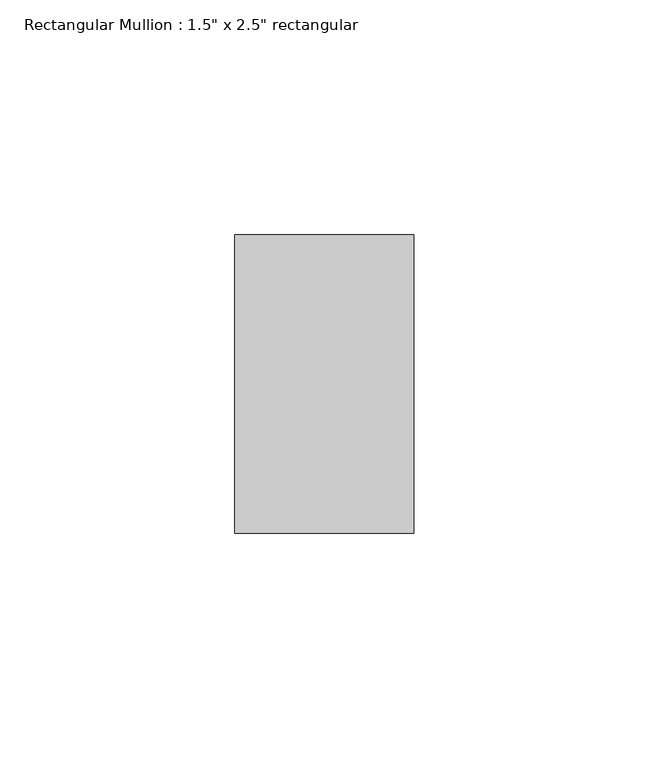
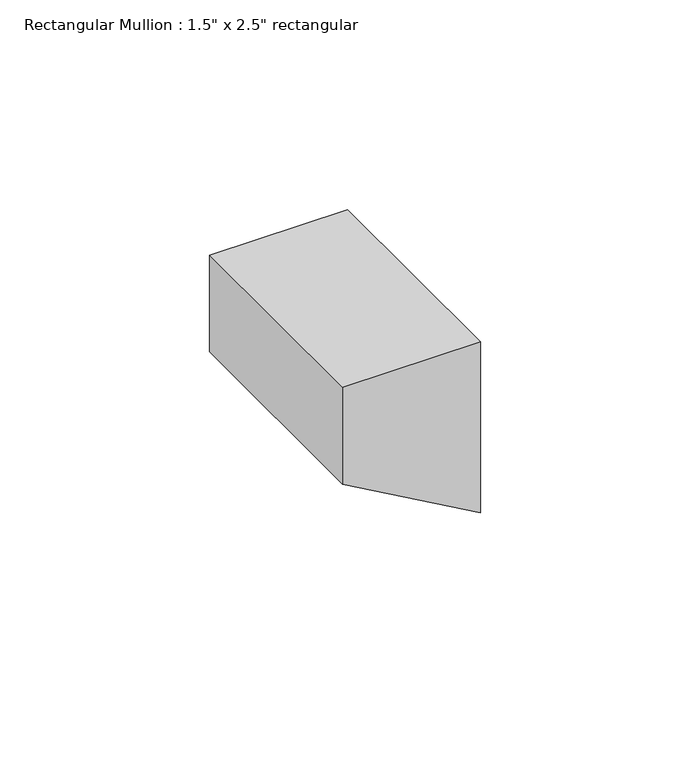
"""IFC4 building model written with IfcOpenShell, lengths in millimetres: member geometry."""

from ifc_helpers import new_model, si_unit, frame, origin, place, context, project, spatial, polyline, outline, extrude, source, transform, mapped, element, save


def member_7b64f847(model_context):
    return source(origin(), model_context, "Body", "SweptSolid", [
        extrude(outline(polyline([(0.0, 0.0), (0.0, -38.1), (-28.1585487, -38.1), (-49.8354067, 0.0), (0.0, 0.0)])), frame((0.0, -31.75, 0.0), z_axis=(0.0, 1.0, 0.0), x_axis=(0.0, 0.0, 1.0)), (0.0, 0.0, 1.0), 63.5),
    ])


if __name__ == "__main__":
    model = new_model("IFC4")
    model_context = context("Model", 3, world=origin())
    ifc_project = project(units=[si_unit("LENGTHUNIT", "METRE", prefix="MILLI")], contexts=[model_context])
    site = spatial("IfcSite", under=ifc_project)
    building = spatial("IfcBuilding", under=site)
    placement = place(None, origin())
    member_shape = member_7b64f847(model_context)
    element("IfcMember", 1, ObjectType="Rectangular Mullion : 1.5\" x 2.5\" rectangular", at=placement, inside=building, context=model_context, shape_type="MappedRepresentation", body=[
        mapped(member_shape, transform((0.0, 0.0, 0.0), x_axis=(1.0, 0.0, 0.0), y_axis=(0.0, 1.0, 0.0), z_axis=(0.0, 0.0, 1.0))),
    ])
    save(model, "model.ifc")

# Revit data of these elements
# Type "Rectangular Mullion : 1.5\" x 2.5\" rectangular"
#   built-in parameter 1007304 = 0.208333 (stored number, unit not read)
#   built-in parameter 1007301 = 0.0625 (stored number, unit not read)
#   built-in parameter 1007300 = 0.0625 (stored number, unit not read)
